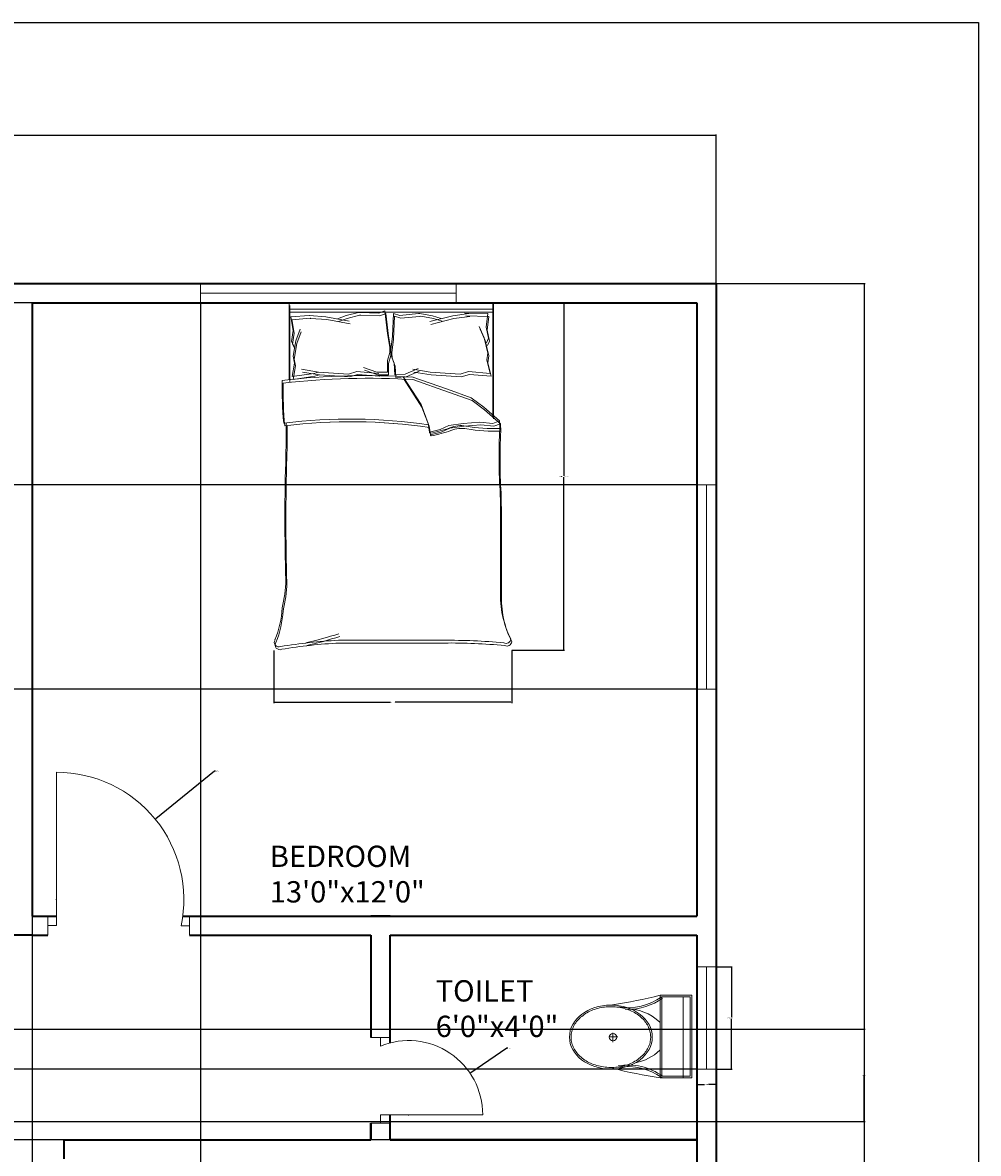
# Model space of a CAD drawing. Units: inches. Extents: x 1861 to 2564, y 1482 to 2317.
# Tile 11 of 11: x 2339 to 2564, y 2051 to 2317. Entities that reach past the tile are written whole.
import ezdxf

# ---------------------------------------------------------------- set-up
doc = ezdxf.new("R2010")
doc.units = ezdxf.units.IN
for name, color, linetype, lineweight in [('A-ANNO-DIMS', 2, 'Continuous', 18), ('A-ANNO-TTLB', 7, 'Continuous', 25), ('A-AREA-IDEN', 7, 'Continuous', 18), ('A-DOOR', 3, 'Continuous', 18), ('A-FLOR-FIXT', 8, 'Continuous', 18), ('A-FURN', 8, 'Continuous', 13), ('A-GLAZ', 4, 'Continuous', 18), ('A-WALL', 7, 'Continuous', 35)]:
    doc.layers.add(name, color=color, linetype=linetype, lineweight=lineweight)
doc.styles.get("Standard").update_dxf_attribs({"font": 'arial.ttf'})
doc.dimstyles.get("Standard").update_dxf_attribs({"dimtxt": 0.18, "dimasz": 0.18, "dimexe": 0.18, "dimexo": 0.0625, "dimgap": 0.09, "dimtad": 0, "dimtih": 1, "dimtoh": 1, "dimdec": 4, "dimzin": 0, "dimdsep": 46, "dimtxsty": 'Standard', "dimcen": 0.09, "dimadec": 0, "dimazin": 0, "dimtfac": 1, "dimtdec": 4, "dimtofl": 0, "dimtmove": 0, "dimatfit": 3, "dimfxl": 1, "dimtolj": 1, "dimtzin": 0, "dimarcsym": 0})

# ---------------------------------------------------------------- blocks, each defined once
blk = doc.blocks.new('A$C31115884')
for p, q in [((257.5, 466.4), (257.5, 523.2)), ((283.1, 497.7), (223.4, 497.7)), ((0, 200), (0, 0)), ((520, 200), (0, 200)), ((10, 190), (10, 10)), ((510, 190), (10, 190)), ((510, 10), (510, 190)), ((520, 0), (520, 200)), ((510, 54.5), (0, 54.5)), ((10, 10), (510, 10)), ((0, 0), (520, 0))]:
    blk.add_line(p, q)
blk.add_circle((255.6, 496.4), 23.6)
for centre, radius, start, end in [((2777.7, -204.6), 2807, 165.4549, 171.71327), ((3237, 905), 2807, 188.28673, 194.5451), ((-294.5, 403.3), 364.7, 324.20913, 9.34987), ((-294.5, 403.3), 374.7, 324.20913, 9.34987), ((805.8, 403.3), 364.7, 170.65013, 215.79087), ((139.5, 406.2), 293.5, 315.84364, 2.65635), ((805.8, 403.3), 374.7, 179.20365, 215.79087), ((383.6, 406.2), 293.5, 190.27735, 224.15636)]:
    blk.add_arc(centre, radius, start, end)
blk.add_ellipse((256.2, 509.9), major_axis=(0, -260.7), ratio=0.772727)
blk.add_open_spline([(256.2, 259.2), (263.1, 259.2), (270, 259.7), (287.8, 262.3), (298.7, 265.1), (319.9, 273.1), (330.2, 278.4), (350.1, 291.1), (359.7, 298.7), (377.7, 315.9), (386.2, 325.5), (401.7, 346.6), (408.8, 358.1), (421.3, 382.5), (426.8, 395.5), (435.9, 422.4), (439.5, 436.4), (444.8, 465.1), (446.5, 479.7), (447.9, 509.2), (447.6, 524), (445, 553.3), (442.7, 567.8), (436.3, 596), (432.1, 609.7), (421.9, 636), (416, 648.6), (402.5, 672.1), (395, 683), (378.6, 703), (369.8, 712.1), (351.1, 728), (341.3, 734.8), (320.9, 746.2), (310.4, 750.7), (288.9, 757.3), (278, 759.4), (256, 761), (245, 760.6), (223.1, 757.2), (212.3, 754.3), (191.1, 746.1), (180.8, 740.7), (160.9, 727.8), (151.4, 720.1), (133.5, 702.7), (125.1, 693), (109.6, 671.7), (102.6, 660.2), (90.2, 635.7), (84.9, 622.7), (76, 595.6), (72.4, 581.6), (67.2, 552.9), (65.6, 538.2), (64.4, 508.8), (64.8, 494), (67.5, 464.7), (69.9, 450.2), (76.6, 422), (80.8, 408.3), (91.1, 382.2), (97.2, 369.7), (110.8, 346.3), (118.4, 335.4), (134.8, 315.6), (143.7, 306.7), (162.4, 290.9), (172.3, 284.2), (192.8, 273), (203.3, 268.6), (224.8, 262.2), (235.8, 260.2), (249.9, 259.3), (253, 259.2), (256.2, 259.2)], degree=3, knots=[0, 0, 0, 0, 0.110105, 0.110105, 0.285049, 0.285049, 0.459994, 0.459994, 0.634938, 0.634938, 0.809882, 0.809882, 0.984827, 0.984827, 1.159771, 1.159771, 1.334715, 1.334715, 1.50966, 1.50966, 1.684604, 1.684604, 1.859549, 1.859549, 2.034493, 2.034493, 2.209437, 2.209437, 2.384382, 2.384382, 2.559326, 2.559326, 2.73427, 2.73427, 2.909215, 2.909215, 3.084159, 3.084159, 3.259103, 3.259103, 3.434048, 3.434048, 3.608992, 3.608992, 3.783936, 3.783936, 3.958881, 3.958881, 4.133825, 4.133825, 4.30877, 4.30877, 4.483714, 4.483714, 4.658658, 4.658658, 4.833603, 4.833603, 5.008547, 5.008547, 5.183491, 5.183491, 5.358436, 5.358436, 5.53338, 5.53338, 5.708324, 5.708324, 5.883269, 5.883269, 6.058213, 6.058213, 6.233158, 6.233158, 6.283185, 6.283185, 6.283185, 6.283185])
blk = doc.blocks.new('WIN-24IN')
for p, q in [((0, 24), (4.5, 24)), ((4.5, 24), (2.25, 24)), ((2.25, 24), (2.25, 0)), ((2.25, 0), (0, 0)), ((0, 0), (4.5, 0))]:
    blk.add_line(p, q)
blk = doc.blocks.new('WIN-60IN')
for p, q in [((0, 4.5), (0, 0)), ((60, 2.25), (60, 4.5)), ((60, 4.5), (60, 0)), ((0, 0), (0, 2.25)), ((0, 2.25), (60, 2.25))]:
    blk.add_line(p, q)
blk = doc.blocks.new('BED-DOUBLE')
for p, q in [((3.48, 63.34), (3.48, 81.45)), ((3.48, 63.34), (3.48, 81.45)), ((51.27, 81.45), (3.48, 81.45)), ((3.48, 79.91), (51.27, 79.91)), ((3.48, 79.91), (51.27, 79.91)), ((3.7, 62.7), (3.7, 80.81)), ((3.7, 62.7), (3.7, 80.81)), ((51.27, 81.45), (51.27, 54.84)), ((51.27, 81.45), (51.27, 54.84)), ((51.27, 81.45), (51.49, 81.45)), ((51.49, 81.45), (51.49, 80.81)), ((51.49, 80.81), (51.49, 54.2)), ((51.49, 80.81), (51.49, 54.2)), ((3.7, 79.27), (51.49, 79.27)), ((3.7, 79.27), (51.49, 79.27)), ((3.9, 78.11), (8.18, 78.44)), ((3.9, 78.11), (8.18, 78.44)), ((3.9, 78.13), (4.47, 74.95)), ((3.9, 78.13), (4.47, 74.95)), ((4.12, 77.49), (4.7, 74.31)), ((4.12, 77.49), (4.7, 74.31)), ((4.13, 77.47), (8.41, 77.8)), ((4.13, 77.47), (8.41, 77.8)), ((8.18, 78.44), (8.29, 78.42)), ((8.18, 78.44), (8.29, 78.42)), ((8.29, 78.42), (12.11, 78.13)), ((8.29, 78.42), (12.11, 78.13)), ((8.41, 77.8), (8.51, 77.78)), ((8.41, 77.8), (8.51, 77.78)), ((8.51, 77.78), (12.34, 77.49)), ((8.51, 77.78), (12.34, 77.49)), ((12.11, 78.13), (17.6, 77.12)), ((12.11, 78.13), (17.6, 77.12)), ((12.34, 77.49), (17.83, 76.48)), ((12.34, 77.49), (17.83, 76.48)), ((14.86, 77.7), (16.88, 78.42)), ((14.86, 77.7), (16.88, 78.42)), ((15.08, 77.06), (17.11, 77.78)), ((15.08, 77.06), (17.11, 77.78)), ((16.88, 78.42), (19.77, 79.14)), ((16.88, 78.42), (19.77, 79.14)), ((17.11, 77.78), (20, 78.5)), ((17.11, 77.78), (20, 78.5)), ((19.77, 79.14), (20.09, 79.14)), ((19.77, 79.14), (20.09, 79.14)), ((20, 78.5), (20.32, 78.5)), ((20, 78.5), (20.32, 78.5)), ((20.09, 79.14), (24.54, 79)), ((20.09, 79.14), (24.54, 79)), ((20.32, 78.5), (24.77, 78.36)), ((20.32, 78.5), (24.77, 78.36)), ((24.54, 79), (25.98, 79.58)), ((24.54, 79), (25.98, 79.58)), ((24.77, 78.36), (26.21, 78.94)), ((24.77, 78.36), (26.21, 78.94)), ((25.98, 79.58), (26.56, 74.23)), ((25.98, 79.58), (26.56, 74.23)), ((26.21, 78.94), (26.79, 73.59)), ((26.21, 78.94), (26.79, 73.59)), ((27.98, 78.95), (27.73, 73.58)), ((27.98, 78.95), (27.73, 73.58)), ((28.21, 78.31), (27.96, 72.94)), ((28.21, 78.31), (27.96, 72.94)), ((29.46, 78.47), (27.98, 78.95)), ((29.46, 78.47), (27.98, 78.95)), ((29.69, 77.83), (28.21, 78.31)), ((29.68, 77.83), (28.21, 78.31)), ((33.88, 78.89), (29.46, 78.47)), ((33.88, 78.89), (29.46, 78.47)), ((34.11, 78.25), (29.68, 77.83)), ((34.11, 78.25), (29.69, 77.83)), ((34.21, 78.91), (33.88, 78.89)), ((34.21, 78.91), (33.88, 78.89)), ((34.43, 78.27), (34.11, 78.25)), ((34.43, 78.27), (34.11, 78.25)), ((37.14, 78.37), (34.21, 78.91)), ((37.14, 78.37), (34.21, 78.91)), ((37.36, 77.73), (34.43, 78.27)), ((37.36, 77.73), (34.43, 78.27)), ((41.92, 78.38), (36.5, 77.02)), ((41.92, 78.38), (36.5, 77.02)), ((42.14, 77.74), (36.72, 76.38)), ((42.14, 77.74), (36.72, 76.38)), ((39.2, 77.77), (37.14, 78.37)), ((39.2, 77.77), (37.14, 78.37)), ((39.43, 77.13), (37.36, 77.73)), ((39.43, 77.13), (37.36, 77.73)), ((45.71, 78.9), (41.92, 78.38)), ((45.71, 78.9), (41.92, 78.38)), ((45.94, 78.26), (42.14, 77.74)), ((45.94, 78.26), (42.14, 77.74)), ((50.11, 78.89), (44.71, 78.99)), ((44.71, 78.99), (45.71, 78.9)), ((50.11, 78.89), (44.71, 78.99)), ((44.71, 78.99), (45.71, 78.9)), ((50.34, 78.25), (44.94, 78.35)), ((44.94, 78.35), (45.94, 78.26)), ((50.34, 78.25), (44.94, 78.35)), ((44.94, 78.35), (45.94, 78.26)), ((50.11, 78.89), (49.73, 75.68)), ((50.11, 78.89), (49.73, 75.68)), ((50.34, 78.25), (49.96, 75.04)), ((50.34, 78.25), (49.96, 75.04)), ((4.47, 74.95), (4.04, 72.35)), ((4.47, 74.95), (4.04, 72.35)), ((5.05, 72.49), (6.06, 75.24)), ((5.05, 72.49), (6.06, 75.24)), ((5.28, 71.85), (6.29, 74.6)), ((5.28, 71.85), (6.29, 74.6)), ((49.31, 73.19), (48.13, 75.87)), ((49.31, 73.19), (48.13, 75.87)), ((49.54, 72.55), (48.36, 75.23)), ((49.54, 72.55), (48.36, 75.23)), ((49.73, 75.68), (50.33, 73.11)), ((49.73, 75.68), (50.33, 73.11)), ((49.96, 75.04), (50.56, 72.47)), ((49.96, 75.04), (50.56, 72.47)), ((4.04, 72.35), (4.62, 71.33)), ((4.04, 72.35), (4.62, 71.33)), ((4.7, 74.31), (4.27, 71.71)), ((4.7, 74.31), (4.27, 71.71)), ((4.27, 71.71), (4.85, 70.69)), ((4.27, 71.71), (4.85, 70.69)), ((4.47, 68.88), (5.05, 72.49)), ((4.47, 68.88), (5.05, 72.49)), ((4.7, 68.24), (5.28, 71.85)), ((4.7, 68.24), (5.28, 71.85)), ((26.56, 74.23), (27.14, 71.04)), ((26.56, 74.23), (27.14, 71.04)), ((26.79, 73.59), (27.37, 70.41)), ((26.79, 73.59), (27.37, 70.41)), ((27.73, 73.58), (27.36, 70.37)), ((27.73, 73.58), (27.36, 70.37)), ((27.96, 72.94), (27.58, 69.73)), ((27.96, 72.94), (27.58, 69.73)), ((50.11, 69.62), (49.31, 73.19)), ((50.11, 69.62), (49.31, 73.19)), ((50.34, 68.98), (49.54, 72.55)), ((50.34, 68.98), (49.54, 72.55)), ((50.33, 73.11), (49.82, 72.06)), ((50.33, 73.11), (49.82, 72.06)), ((50.56, 72.47), (50.04, 71.42)), ((50.56, 72.47), (50.04, 71.42)), ((27.14, 69.74), (26.56, 67.86)), ((27.14, 69.74), (26.56, 67.86)), ((27.37, 69.1), (26.79, 67.22)), ((27.37, 69.1), (26.79, 67.22)), ((27.14, 71.04), (27.14, 69.74)), ((27.14, 71.04), (27.14, 69.74)), ((27.36, 70.37), (27.44, 69.07)), ((27.36, 70.37), (27.44, 69.07)), ((27.37, 70.41), (27.37, 69.1)), ((27.37, 70.41), (27.37, 69.1)), ((27.44, 69.07), (28.13, 67.23)), ((27.44, 69.07), (28.13, 67.23)), ((27.58, 69.73), (27.67, 68.43)), ((27.58, 69.73), (27.67, 68.43)), ((49.92, 68.01), (50.11, 69.62)), ((49.92, 68.01), (50.11, 69.62)), ((4.18, 64.1), (4.76, 67.29)), ((4.18, 64.1), (4.76, 67.29)), ((4.41, 63.46), (4.99, 66.65)), ((4.41, 63.46), (4.99, 66.65)), ((4.76, 67.29), (4.47, 68.88)), ((4.76, 67.29), (4.47, 68.88)), ((4.99, 66.65), (4.7, 68.24)), ((4.99, 66.65), (4.7, 68.24)), ((26.56, 67.86), (26.56, 65.18)), ((26.56, 67.86), (26.56, 65.18)), ((26.79, 67.22), (26.79, 64.54)), ((26.79, 67.22), (26.79, 64.54)), ((27.67, 68.43), (28.36, 66.59)), ((27.67, 68.43), (28.36, 66.59)), ((28.13, 67.23), (28.3, 64.55)), ((28.13, 67.23), (28.3, 64.55)), ((28.36, 66.59), (28.53, 63.91)), ((28.36, 66.59), (28.53, 63.91)), ((50.7, 64.87), (49.92, 68.01)), ((50.7, 64.87), (49.92, 68.01)), ((50.15, 67.37), (50.34, 68.98)), ((50.15, 67.37), (50.34, 68.98)), ((50.93, 64.23), (50.15, 67.37)), ((50.93, 64.23), (50.15, 67.37)), ((9.28, 64.83), (4.18, 64.1)), ((9.28, 64.83), (4.18, 64.1)), ((9.51, 64.19), (4.41, 63.46)), ((9.51, 64.19), (4.41, 63.46)), ((6.38, 65.82), (10.41, 65.15)), ((6.38, 65.82), (10.41, 65.15)), ((6.61, 65.18), (10.64, 64.51)), ((6.61, 65.18), (10.64, 64.51)), ((10.41, 65.15), (9.28, 64.83)), ((10.41, 65.15), (9.28, 64.83)), ((10.64, 64.51), (9.51, 64.19)), ((10.64, 64.51), (9.51, 64.19)), ((10.41, 65.15), (17.42, 64.72)), ((10.41, 65.15), (17.42, 64.72)), ((10.64, 64.51), (17.65, 64.08)), ((10.64, 64.51), (17.65, 64.08)), ((17.42, 64.72), (19.38, 65.28)), ((17.42, 64.72), (19.38, 65.28)), ((17.65, 64.08), (19.61, 64.64)), ((17.65, 64.08), (19.61, 64.64)), ((19.38, 65.28), (24.52, 64.87)), ((19.38, 65.28), (24.52, 64.87)), ((19.61, 64.64), (24.75, 64.23)), ((19.61, 64.64), (24.74, 64.23)), ((24.1, 65.18), (20.96, 66.27)), ((24.1, 65.18), (20.96, 66.27)), ((24.33, 64.54), (21.19, 65.63)), ((24.33, 64.54), (21.19, 65.63)), ((26.56, 65.18), (24.1, 65.18)), ((26.56, 65.18), (24.1, 65.18)), ((26.79, 64.54), (24.33, 64.54)), ((26.79, 64.54), (24.33, 64.54)), ((28.3, 64.55), (30.75, 64.71)), ((28.3, 64.55), (30.75, 64.71)), ((28.53, 63.91), (30.98, 64.07)), ((28.53, 63.91), (30.98, 64.07)), ((30.26, 64.06), (34.45, 57.57)), ((30.26, 64.06), (34.45, 57.57)), ((30.75, 64.71), (33.82, 65.99)), ((30.75, 64.71), (33.82, 65.99)), ((30.98, 64.07), (34.05, 65.35)), ((30.98, 64.07), (34.05, 65.35)), ((40.65, 61.13), (32.31, 64.06)), ((40.64, 61.13), (32.31, 64.06)), ((32.56, 65.82), (36.6, 65.15)), ((32.57, 65.82), (36.6, 65.15)), ((32.79, 65.18), (36.83, 64.51)), ((32.79, 65.18), (36.83, 64.51)), ((36.6, 65.15), (43.61, 64.72)), ((36.6, 65.15), (43.61, 64.72)), ((36.83, 64.51), (43.84, 64.08)), ((36.83, 64.51), (43.84, 64.08)), ((43.61, 64.72), (45.57, 65.28)), ((43.61, 64.72), (45.57, 65.28)), ((43.84, 64.08), (45.8, 64.64)), ((43.84, 64.08), (45.8, 64.64)), ((45.57, 65.28), (50.7, 64.87)), ((45.57, 65.28), (50.7, 64.87)), ((45.8, 64.64), (50.93, 64.23)), ((45.8, 64.64), (50.93, 64.23)), ((30.49, 63.42), (34.68, 56.93)), ((30.49, 63.42), (34.68, 56.93)), ((40.87, 60.49), (32.54, 63.42)), ((40.87, 60.49), (32.54, 63.42)), ((46.22, 59.12), (40.64, 61.13)), ((46.22, 59.12), (40.65, 61.13)), ((46.45, 58.48), (40.87, 60.49)), ((46.45, 58.48), (40.87, 60.49)), ((49.16, 56.95), (46.22, 59.12)), ((49.16, 56.95), (46.22, 59.12)), ((49.39, 56.31), (46.45, 58.48)), ((49.39, 56.31), (46.45, 58.48)), ((34.45, 57.57), (36.15, 53.08)), ((34.45, 57.57), (36.15, 53.08)), ((34.68, 56.93), (36.38, 52.44)), ((34.68, 56.93), (36.38, 52.44)), ((52.87, 53.7), (49.16, 56.95)), ((52.87, 53.7), (49.16, 56.95)), ((53.1, 53.06), (49.39, 56.31)), ((53.1, 53.06), (49.39, 56.31)), ((44.36, 53.08), (48.23, 53.39)), ((44.36, 53.08), (48.23, 53.39)), ((48.23, 53.39), (51.33, 53.08)), ((48.23, 53.39), (51.33, 53.08)), ((51.33, 53.08), (52.87, 53.7)), ((51.33, 53.08), (52.87, 53.7)), ((52.95, 51.95), (52.87, 53.7, 3.87)), ((52.95, 51.95), (52.87, 53.7, 3.87)), ((36.15, 53.08), (36.46, 51.07)), ((36.15, 53.08), (36.46, 51.07)), ((36.38, 52.44), (36.69, 50.43)), ((36.38, 52.44), (36.69, 50.43)), ((36.46, 51.07), (38.94, 51.69)), ((36.46, 51.07), (38.94, 51.69)), ((36.69, 50.43), (39.17, 51.05)), ((36.69, 50.43), (39.17, 51.05)), ((38.94, 51.69), (40.95, 52.62)), ((38.94, 51.69), (40.95, 52.62)), ((39.17, 51.05), (41.18, 51.98)), ((39.17, 51.05), (41.18, 51.98)), ((40.95, 52.62), (44.36, 53.08)), ((40.95, 52.62), (44.36, 53.08)), ((41.18, 51.98), (44.59, 52.44)), ((41.18, 51.98), (44.59, 52.44)), ((44.59, 52.44), (48.46, 52.75)), ((44.59, 52.44), (48.46, 52.75)), ((48.46, 52.75), (51.56, 52.44)), ((48.46, 52.75), (51.56, 52.44)), ((51.56, 52.44), (53.1, 53.06)), ((51.56, 52.44), (53.1, 53.06)), ((53.18, 51.32), (53.1, 53.06, 3.87)), ((53.18, 51.32), (53.1, 53.06, 3.87)), ((15.06, 2.2), (39.68, 2.2)), ((15.06, 2.2), (39.68, 2.2)), ((15.29, 1.56), (39.91, 1.56)), ((15.29, 1.56), (39.91, 1.56))]:
    blk.add_line(p, q)
for centre, radius, start, end in [((21.36, -100.61), 164.97, 86.0865, 96.7821), ((21.36, -100.61), 164.97, 86.0865, 96.7821), ((21.59, -101.25), 164.97, 86.0865, 96.7821), ((21.59, -101.25), 164.97, 86.0865, 96.7821), ((85.16, 61.35), 83.31, 178.7218, 185.604), ((85.16, 61.35), 83.31, 178.7218, 185.604), ((85.39, 60.71), 83.31, 178.7218, 185.604), ((85.39, 60.71), 83.31, 178.7218, 185.604), ((17.76, -74.87), 129.02, 81.7845, 96.9006), ((17.76, -74.87), 129.02, 81.7845, 96.9006), ((17.99, -75.51), 129.02, 81.7845, 96.9006), ((17.98, -75.51), 129.02, 81.7845, 96.9006), ((-167.31, 50.27), 170.11, 358.4762, 1.0082), ((-167.31, 50.27), 170.11, 358.4762, 1.0082), ((-167.08, 49.63), 170.11, 358.4762, 1.0082), ((-167.08, 49.63), 170.11, 358.4762, 1.0082), ((36.64, 51.01), 0.185, 160.2464, 271.1377), ((36.64, 51.01), 0.185, 160.2464, 271.1377), ((31.15, 79.96), 29.65, 280.6617, 289.8806), ((31.15, 79.96), 29.65, 280.6617, 289.8806), ((31.38, 79.32), 29.65, 280.6617, 289.8806), ((31.38, 79.32), 29.65, 280.6617, 289.8806), ((43.74, 46.38), 6.22, 78.6608, 113.7384), ((43.74, 46.38), 6.22, 78.6608, 113.7384), ((43.97, 45.74), 6.22, 78.6608, 113.7384), ((43.97, 45.74), 6.22, 78.6608, 113.7384), ((51.33, 88.1), 36.18, 259.8763, 272.5657), ((51.33, 88.1), 36.18, 259.8763, 272.5657), ((51.56, 87.46), 36.18, 259.8763, 272.5657), ((51.56, 87.46), 36.18, 259.8763, 272.5657), ((182.27, 45.13), 129.5, 176.9791, 183.8365), ((182.27, 45.13), 129.5, 176.9791, 183.8365), ((182.5, 44.49), 129.5, 176.9791, 183.8365), ((182.49, 44.49), 129.5, 176.9791, 183.8365), ((36.87, 50.37), 0.185, 160.2464, 271.1377), ((36.87, 50.37), 0.185, 160.2464, 271.1377), ((484.82, 30.83), 482.31, 178.2277, 181.7185), ((484.82, 30.83), 482.31, 178.2277, 181.7185), ((485.05, 30.19), 482.31, 178.2277, 181.7185), ((485.05, 30.19), 482.31, 178.2277, 181.7185), ((-4508.74, 13.62), 4561.86, 0.00217, 0.28689), ((-4508.74, 13.62), 4561.86, 0.00217, 0.28689), ((-4508.51, 12.98), 4561.86, 0.00217, 0.28689), ((-4508.51, 12.98), 4561.86, 0.00217, 0.28689), ((-26.9, 16.93), 29.63, 346.0648, 358.9113), ((-26.9, 16.93), 29.63, 346.0648, 358.9113), ((-26.67, 16.29), 29.63, 346.0648, 358.9113), ((-26.67, 16.29), 29.63, 346.0648, 358.9113), ((76.16, 12.78), 23.07, 177.4714, 206.4681), ((76.16, 12.78), 23.07, 177.4714, 206.4681), ((76.39, 12.14), 23.07, 177.4714, 206.4681), ((76.39, 12.14), 23.07, 177.4714, 206.4681), ((-21.66, 11.17), 23.56, 337.9751, 356.652), ((-21.66, 11.17), 23.56, 337.9751, 356.652), ((-21.43, 10.53), 23.56, 337.9751, 356.652), ((-21.43, 10.53), 23.56, 337.9751, 356.652), ((-17.22, 105.16), 106.46, 283.3832, 287.7053), ((-17.22, 105.16), 106.46, 283.3832, 287.7053), ((-16.99, 104.52), 106.46, 283.3832, 287.7053), ((-16.99, 104.52), 106.46, 283.3832, 287.7053), ((1.09, 1.73), 1.09, 146.1736, 293.4781), ((1.09, 1.73), 1.09, 146.1736, 293.4781), ((1.32, 1.09), 1.09, 146.1736, 293.4781), ((1.32, 1.09), 1.09, 146.1736, 293.4781), ((21.43, -119.39), 121.76, 92.9958, 99.4091), ((21.43, -119.39), 121.76, 92.9958, 99.4091), ((21.66, -120.03), 121.76, 92.9958, 99.4091), ((21.66, -120.03), 121.76, 92.9958, 99.4091), ((41.15, -130.83), 133.04, 84.4998, 90.6351), ((41.15, -130.83), 133.04, 84.4998, 90.6351), ((41.38, -131.47), 133.04, 84.4998, 90.6351), ((41.38, -131.47), 133.04, 84.4998, 90.6351), ((54.41, 2.58), 1.1, 242.6588, 356.02), ((54.41, 2.58), 1.1, 242.6588, 356.02), ((54.64, 1.94), 1.1, 242.6588, 356.02), ((54.64, 1.94), 1.1, 242.6588, 356.02)]:
    blk.add_arc(centre, radius, start, end)
blk = doc.blocks.new('*D12')
at = {"layer": 'A-ANNO-DIMS', "color": 0, "lineweight": -2, "transparency": 16777216}
for p, q in [((2454.34, 2250.89), (2466.69, 2250.89)), ((2466.51, 2250.71), (2466.51, 2210.29)), ((2466.51, 2169.52), (2466.51, 2209.93)), ((2454.34, 2169.34), (2466.69, 2169.34))]:
    blk.add_line(p, q, dxfattribs=at)
at = {"layer": 'A-ANNO-DIMS', "color": 0, "transparency": 16777216}
for points in [[(2466.48, 2250.71), (2466.54, 2250.71), (2466.51, 2250.89)], [(2466.48, 2169.52), (2466.54, 2169.52), (2466.51, 2169.34)]]:
    blk.add_solid(points, dxfattribs=at)
at = {"layer": 'Defpoints', "color": 0, "transparency": 16777216}
for p in [(2454.28, 2250.89), (2466.51, 2250.89), (2454.28, 2169.34)]:
    blk.add_point(p, dxfattribs=at)
at = {"layer": 'A-ANNO-DIMS', "color": 0, "transparency": 16777216, "insert": (2466.51, 2210.11), "char_height": 0.18, "attachment_point": 5}
blk.add_mtext('\\A1;DOUBLE BED 82 TYP.', dxfattribs=at)
blk = doc.blocks.new('*D13')
at = {"layer": 'A-ANNO-DIMS', "color": 0, "lineweight": -2, "transparency": 16777216}
for p, q in [((2398.45, 2169.27), (2398.45, 2156.92)), ((2454.28, 2169.27), (2454.28, 2156.92)), ((2398.63, 2157.1), (2425.84, 2157.1)), ((2454.1, 2157.1), (2426.89, 2157.1))]:
    blk.add_line(p, q, dxfattribs=at)
at = {"layer": 'A-ANNO-DIMS', "color": 0, "transparency": 16777216}
for points in [[(2398.63, 2157.13), (2398.63, 2157.07), (2398.45, 2157.1)], [(2454.1, 2157.13), (2454.1, 2157.07), (2454.28, 2157.1)]]:
    blk.add_solid(points, dxfattribs=at)
at = {"layer": 'Defpoints', "color": 0, "transparency": 16777216}
for p in [(2398.45, 2169.34), (2454.28, 2169.34), (2454.28, 2157.1)]:
    blk.add_point(p, dxfattribs=at)
at = {"layer": 'A-ANNO-DIMS', "color": 0, "transparency": 16777216, "insert": (2426.37, 2157.1), "char_height": 0.18, "attachment_point": 5}
blk.add_mtext('\\A1;56 TYP.', dxfattribs=at)
blk = doc.blocks.new('*D16')
at = {"layer": 'A-ANNO-DIMS', "color": 0, "lineweight": -2, "transparency": 16777216}
for p, q in [((2502.3, 2094.96), (2506.02, 2094.96)), ((2505.84, 2094.78), (2505.84, 2083.14)), ((2505.84, 2071.14), (2505.84, 2082.77)), ((2502.3, 2070.96), (2506.02, 2070.96))]:
    blk.add_line(p, q, dxfattribs=at)
at = {"layer": 'A-ANNO-DIMS', "color": 0, "transparency": 16777216}
for points in [[(2505.81, 2094.78), (2505.87, 2094.78), (2505.84, 2094.96)], [(2505.81, 2071.14), (2505.87, 2071.14), (2505.84, 2070.96)]]:
    blk.add_solid(points, dxfattribs=at)
at = {"layer": 'Defpoints', "color": 0, "transparency": 16777216}
for p in [(2502.24, 2094.96), (2505.84, 2094.96), (2502.24, 2070.96)]:
    blk.add_point(p, dxfattribs=at)
at = {"layer": 'A-ANNO-DIMS', "color": 0, "transparency": 16777216, "insert": (2505.84, 2082.96), "char_height": 0.18, "attachment_point": 5}
blk.add_mtext('\\A1;WINDOW 24 TYP.', dxfattribs=at)
blk = doc.blocks.new('*D17')
at = {"layer": 'A-ANNO-DIMS', "color": 0, "lineweight": -2, "transparency": 16777216}
for p, q in [((2497.74, 2070.89), (2497.74, 2067.18)), ((2502.24, 2070.89), (2502.24, 2067.18)), ((2497.92, 2067.36), (2499.53, 2067.36)), ((2502.06, 2067.36), (2500.45, 2067.36))]:
    blk.add_line(p, q, dxfattribs=at)
at = {"layer": 'A-ANNO-DIMS', "color": 0, "transparency": 16777216}
for points in [[(2497.92, 2067.39), (2497.92, 2067.33), (2497.74, 2067.36)], [(2502.06, 2067.39), (2502.06, 2067.33), (2502.24, 2067.36)]]:
    blk.add_solid(points, dxfattribs=at)
at = {"layer": 'Defpoints', "color": 0, "transparency": 16777216}
for p in [(2497.74, 2070.96), (2502.24, 2070.96), (2502.24, 2067.36)]:
    blk.add_point(p, dxfattribs=at)
at = {"layer": 'A-ANNO-DIMS', "color": 0, "transparency": 16777216, "insert": (2499.99, 2067.36), "char_height": 0.18, "attachment_point": 5}
blk.add_mtext('\\A1;5 TYP.', dxfattribs=at)
blk = doc.blocks.new('*D34')
at = {"layer": 'A-ANNO-DIMS', "color": 0, "lineweight": -2, "transparency": 16777216}
for p, q in [((1927.74, 2255.45), (1927.74, 2290.37)), ((1927.92, 2290.19), (2214.59, 2290.19)), ((2502.06, 2290.19), (2215.38, 2290.19)), ((2502.24, 2255.45), (2502.24, 2290.37))]:
    blk.add_line(p, q, dxfattribs=at)
at = {"layer": 'A-ANNO-DIMS', "color": 0, "transparency": 16777216}
for points in [[(1927.92, 2290.22), (1927.92, 2290.16), (1927.74, 2290.19)], [(2502.06, 2290.22), (2502.06, 2290.16), (2502.24, 2290.19)]]:
    blk.add_solid(points, dxfattribs=at)
at = {"layer": 'Defpoints', "color": 0, "transparency": 16777216}
for p in [(2502.24, 2290.19), (1927.74, 2255.39), (2502.24, 2255.39)]:
    blk.add_point(p, dxfattribs=at)
at = {"layer": 'A-ANNO-DIMS', "color": 0, "transparency": 16777216, "insert": (2214.99, 2290.19), "char_height": 0.18, "attachment_point": 5}
blk.add_mtext('\\A1;574.5', dxfattribs=at)
blk = doc.blocks.new('*D38')
at = {"layer": 'A-ANNO-DIMS', "color": 0, "lineweight": -2, "transparency": 16777216}
for p, q in [((2341.74, 2250.82), (2341.74, 1545.6)), ((2381.24, 2250.82), (2381.24, 1545.6)), ((2341.92, 1545.78), (2361.16, 1545.78)), ((2381.06, 1545.78), (2361.81, 1545.78))]:
    blk.add_line(p, q, dxfattribs=at)
at = {"layer": 'A-ANNO-DIMS', "color": 0, "transparency": 16777216}
for points in [[(2341.92, 1545.81), (2341.92, 1545.75), (2341.74, 1545.78)], [(2381.06, 1545.81), (2381.06, 1545.75), (2381.24, 1545.78)]]:
    blk.add_solid(points, dxfattribs=at)
at = {"layer": 'Defpoints', "color": 0, "transparency": 16777216}
for p in [(2341.74, 2250.89), (2381.24, 2250.89), (2381.24, 1545.78)]:
    blk.add_point(p, dxfattribs=at)
at = {"layer": 'A-ANNO-DIMS', "color": 0, "transparency": 16777216, "insert": (2361.49, 1545.78), "char_height": 0.18, "attachment_point": 5}
blk.add_mtext('\\A1;39.5', dxfattribs=at)
blk = doc.blocks.new('*D45')
at = {"layer": 'A-ANNO-DIMS', "color": 0, "lineweight": -2, "transparency": 16777216}
for p, q in [((2502.3, 2255.39), (2537.22, 2255.39)), ((2537.04, 2255.21), (2537.04, 1951.82)), ((2537.04, 1648.07), (2537.04, 1951.45)), ((2473.32, 1647.89), (2537.22, 1647.89))]:
    blk.add_line(p, q, dxfattribs=at)
at = {"layer": 'A-ANNO-DIMS', "color": 0, "transparency": 16777216}
for points in [[(2537.01, 2255.21), (2537.07, 2255.21), (2537.04, 2255.39)], [(2537.01, 1648.07), (2537.07, 1648.07), (2537.04, 1647.89)]]:
    blk.add_solid(points, dxfattribs=at)
at = {"layer": 'Defpoints', "color": 0, "transparency": 16777216}
for p in [(2502.24, 2255.39), (2537.04, 2255.39), (2473.26, 1647.89)]:
    blk.add_point(p, dxfattribs=at)
at = {"layer": 'A-ANNO-DIMS', "color": 0, "transparency": 16777216, "insert": (2537.04, 1951.64), "char_height": 0.18, "attachment_point": 5}
blk.add_mtext('\\A1;607.5', dxfattribs=at)
blk = doc.blocks.new('*D60')
at = {"layer": 'A-ANNO-DIMS', "color": 0, "lineweight": -2, "transparency": 16777216}
for p, q in [((2497.68, 2208.17), (1892.76, 2208.17)), ((1892.94, 2207.99), (1892.94, 2184.35)), ((1892.94, 2160.35), (1892.94, 2183.99)), ((2497.68, 2160.17), (1892.76, 2160.17))]:
    blk.add_line(p, q, dxfattribs=at)
at = {"layer": 'A-ANNO-DIMS', "color": 0, "transparency": 16777216}
for points in [[(1892.91, 2207.99), (1892.97, 2207.99), (1892.94, 2208.17)], [(1892.91, 2160.35), (1892.97, 2160.35), (1892.94, 2160.17)]]:
    blk.add_solid(points, dxfattribs=at)
at = {"layer": 'Defpoints', "color": 0, "transparency": 16777216}
for p in [(1892.94, 2208.17), (2497.74, 2208.17), (2497.74, 2160.17)]:
    blk.add_point(p, dxfattribs=at)
at = {"layer": 'A-ANNO-DIMS', "color": 0, "transparency": 16777216, "insert": (1892.94, 2184.17), "char_height": 0.18, "attachment_point": 5}
blk.add_mtext('\\A1;48', dxfattribs=at)
blk = doc.blocks.new('*D61')
at = {"layer": 'A-ANNO-DIMS', "color": 0, "lineweight": -2, "transparency": 16777216}
for p, q in [((2008.8, 2080.33), (2537.22, 2080.33)), ((2537.04, 2080.15), (2537.04, 2069.66)), ((2537.04, 2058.82), (2537.04, 2069.3)), ((2008.8, 2058.64), (2537.22, 2058.64))]:
    blk.add_line(p, q, dxfattribs=at)
at = {"layer": 'A-ANNO-DIMS', "color": 0, "transparency": 16777216}
for points in [[(2537.01, 2080.15), (2537.07, 2080.15), (2537.04, 2080.33)], [(2537.01, 2058.82), (2537.07, 2058.82), (2537.04, 2058.64)]]:
    blk.add_solid(points, dxfattribs=at)
at = {"layer": 'Defpoints', "color": 0, "transparency": 16777216}
for p in [(2008.74, 2080.33), (2537.04, 2080.33), (2008.74, 2058.64)]:
    blk.add_point(p, dxfattribs=at)
at = {"layer": 'A-ANNO-DIMS', "color": 0, "transparency": 16777216, "insert": (2537.04, 2069.48), "char_height": 0.18, "attachment_point": 5}
blk.add_mtext('\\A1;21.693', dxfattribs=at)
blk = doc.blocks.new('*D63')
at = {"layer": 'A-ANNO-DIMS', "color": 0, "lineweight": -2, "transparency": 16777216}
for p, q in [((2497.68, 2250.89), (1892.76, 2250.89)), ((1892.94, 2250.71), (1892.94, 2229.71)), ((1892.94, 2208.35), (1892.94, 2229.35)), ((2497.68, 2208.17), (1892.76, 2208.17))]:
    blk.add_line(p, q, dxfattribs=at)
at = {"layer": 'A-ANNO-DIMS', "color": 0, "transparency": 16777216}
for points in [[(1892.91, 2250.71), (1892.97, 2250.71), (1892.94, 2250.89)], [(1892.91, 2208.35), (1892.97, 2208.35), (1892.94, 2208.17)]]:
    blk.add_solid(points, dxfattribs=at)
at = {"layer": 'Defpoints', "color": 0, "transparency": 16777216}
for p in [(2497.74, 2250.89), (1892.94, 2208.17), (2497.74, 2208.17)]:
    blk.add_point(p, dxfattribs=at)
at = {"layer": 'A-ANNO-DIMS', "color": 0, "transparency": 16777216, "insert": (1892.94, 2229.53), "char_height": 0.18, "attachment_point": 5}
blk.add_mtext('\\A1;42.71', dxfattribs=at)
blk = doc.blocks.new('*D64')
at = {"layer": 'A-ANNO-DIMS', "color": 0, "lineweight": -2, "transparency": 16777216}
for p, q in [((2497.68, 2070.96), (1892.76, 2070.96)), ((1892.94, 2070.78), (1892.94, 2062.85)), ((1892.94, 2054.57), (1892.94, 2062.49)), ((2497.68, 2054.39), (1892.76, 2054.39))]:
    blk.add_line(p, q, dxfattribs=at)
at = {"layer": 'A-ANNO-DIMS', "color": 0, "transparency": 16777216}
for points in [[(1892.91, 2070.78), (1892.97, 2070.78), (1892.94, 2070.96)], [(1892.91, 2054.57), (1892.97, 2054.57), (1892.94, 2054.39)]]:
    blk.add_solid(points, dxfattribs=at)
at = {"layer": 'Defpoints', "color": 0, "transparency": 16777216}
for p in [(2497.74, 2070.96), (1892.94, 2054.39), (2497.74, 2054.39)]:
    blk.add_point(p, dxfattribs=at)
at = {"layer": 'A-ANNO-DIMS', "color": 0, "transparency": 16777216, "insert": (1892.94, 2062.67), "char_height": 0.18, "attachment_point": 5}
blk.add_mtext('\\A1;16.57', dxfattribs=at)
blk = doc.blocks.new('*D78')
at = {"layer": 'A-ANNO-DIMS', "color": 0, "lineweight": -2, "transparency": 16777216}
for p, q in [((2384.56, 2140.93), (2370.77, 2129.73)), ((2384.74, 2140.93), (2384.56, 2140.93)), ((2347.33, 2110.77), (2347.51, 2110.77)), ((2347.42, 2110.68), (2347.42, 2110.86))]:
    blk.add_line(p, q, dxfattribs=at)
at = {"layer": 'A-ANNO-DIMS', "color": 0, "transparency": 16777216}
blk.add_solid([(2370.75, 2129.75), (2370.79, 2129.71), (2370.63, 2129.62)], dxfattribs=at)
at = {"layer": 'Defpoints', "color": 0, "transparency": 16777216}
for p in [(2370.63, 2129.62), (2347.42, 2110.77)]:
    blk.add_point(p, dxfattribs=at)
at = {"layer": 'A-ANNO-DIMS', "color": 0, "transparency": 16777216, "insert": (2385.15, 2140.93), "char_height": 0.18, "attachment_point": 5}
blk.add_mtext('\\A1;R29.9', dxfattribs=at)
blk = doc.blocks.new('*D91')
at = {"layer": 'A-ANNO-DIMS', "color": 0, "lineweight": -2, "transparency": 16777216}
for p, q in [((2453.17, 2075.86), (2444.65, 2070.1)), ((2453.35, 2075.86), (2453.17, 2075.86)), ((2429.97, 2060.24), (2430.15, 2060.24)), ((2430.06, 2060.15), (2430.06, 2060.33))]:
    blk.add_line(p, q, dxfattribs=at)
at = {"layer": 'A-ANNO-DIMS', "color": 0, "transparency": 16777216}
blk.add_solid([(2444.63, 2070.13), (2444.67, 2070.08), (2444.5, 2070)], dxfattribs=at)
at = {"layer": 'Defpoints', "color": 0, "transparency": 16777216}
for p in [(2444.5, 2070), (2430.06, 2060.24)]:
    blk.add_point(p, dxfattribs=at)
at = {"layer": 'A-ANNO-DIMS', "color": 0, "transparency": 16777216, "insert": (2453.83, 2075.86), "char_height": 0.18, "attachment_point": 5}
blk.add_mtext('\\A1;R17.43', dxfattribs=at)

msp = doc.modelspace()

# ---------------------------------------------------------------- linework, layer by layer
at = {"layer": 'A-ANNO-TTLB'}
msp.add_lwpolyline([(1861.1332, 2316.6589), (2563.8077, 2316.6589), (2563.8077, 1482.0728), (1861.1332, 1482.0728)], close=True, dxfattribs=at)
at = {"layer": 'A-DOOR'}
for p, q in [((2347.422, 2104.6664), (2347.422, 2140.6664)), ((2345.422, 2106.8854), (2345.422, 2103.5496)), ((2378.6849, 2106.8854), (2378.6849, 2102.3854)), ((2345.422, 2102.3854), (2345.422, 2104.6664)), ((2345.422, 2104.6664), (2347.422, 2104.6664)), ((2345.422, 2103.5496), (2345.422, 2102.3854)), ((2378.6849, 2104.6354), (2376.6849, 2104.6354)), ((2378.6849, 2102.3854), (2378.6849, 2104.6354)), ((2421.2393, 2078.3854), (2425.7393, 2078.3854)), ((2425.7393, 2078.3854), (2423.4893, 2078.3854)), ((2423.4893, 2078.3854), (2423.4893, 2076.3854)), ((2423.4893, 2058.2408), (2423.4893, 2060.2408)), ((2423.4893, 2060.2408), (2447.4893, 2060.2408)), ((2421.2393, 2058.2408), (2425.7393, 2058.2408)), ((2425.7393, 2058.2408), (2421.2393, 2058.2408)), ((2421.2393, 2058.2408), (2423.4893, 2058.2408))]:
    msp.add_line(p, q, dxfattribs=at)
for centre, radius, start, end in [((2347.422, 2110.7678), 29.8986, 348.164205, 90), ((2430.0591, 2060.2408), 17.4302, 360, 112.143263)]:
    msp.add_arc(centre, radius, start, end, dxfattribs=at)
at = {"layer": 'A-GLAZ'}
for p, q in [((2497.7393, 2208.1728), (2502.2393, 2208.1728)), ((2502.2393, 2208.1728), (2499.9893, 2208.1728)), ((2499.9893, 2208.1728), (2499.9893, 2160.1728)), ((2499.9893, 2160.1728), (2497.7393, 2160.1728)), ((2497.7393, 2160.1728), (2502.2393, 2160.1728))]:
    msp.add_line(p, q, dxfattribs=at)
at = {"layer": 'A-WALL'}
for p, q in [((1927.7393, 2255.3854), (2502.2393, 2255.3854)), ((2502.2393, 2255.3854), (2502.2393, 1700.3854)), ((2341.7393, 2250.8854), (2341.7393, 2106.8854)), ((2341.7393, 2250.8854), (2497.7393, 2250.8854)), ((2497.7393, 2250.8854), (2497.7393, 2106.8854)), ((2341.7393, 2106.8854), (2347.422, 2106.8854)), ((2377.0674, 2106.8854), (2497.7393, 2106.8854)), ((2425.7393, 2106.8854), (2421.2393, 2106.8854)), ((2341.7393, 2102.3854), (2337.2393, 2102.3854)), ((2341.7393, 2102.3854), (2345.422, 2102.3854)), ((2378.6849, 2102.3854), (2421.2393, 2102.3854)), ((2421.2393, 2102.3854), (2421.2393, 2078.3854)), ((2425.7393, 2077.1272), (2425.7393, 2102.3854)), ((2425.7393, 2102.3854), (2497.7393, 2102.3854)), ((2497.7393, 2102.3854), (2497.7393, 1905.8854)), ((2425.7393, 2054.3854), (2425.7393, 2060.2408)), ((2421.2393, 2054.3854), (2421.2393, 2058.2408)), ((2421.2393, 2058.2408), (2421.2393, 2054.3854)), ((2349.2393, 2049.8854), (2349.2393, 2054.3854)), ((2349.2393, 2054.3854), (2378.6849, 2054.3854)), ((2378.6849, 2054.3854), (2421.2393, 2054.3854)), ((2497.7393, 2054.3854), (2425.7393, 2054.3854)), ((2425.7393, 2054.3854), (2497.7393, 2054.3854))]:
    msp.add_line(p, q, dxfattribs=at)

# ---------------------------------------------------------------- block references
at = {"layer": 'A-FLOR-FIXT', "xscale": 0.0372717239612423, "yscale": 0.0372717239612423, "zscale": 0.0372717239612423, "rotation": 89.99999999999999}
msp.add_blockref('A$C31115884', (2496.5571, 2068.9422), dxfattribs=at)
at = {"layer": 'A-FURN'}
msp.add_blockref('BED-DOUBLE', (2398.54, 2169.44), dxfattribs=at)
at = {"layer": 'A-GLAZ'}
for name, p in [('WIN-60IN', (2381.2382, 2250.89)), ('WIN-24IN', (2497.74, 2070.96))]:
    msp.add_blockref(name, p, dxfattribs=at)

# ---------------------------------------------------------------- texts
at = {"layer": 'A-AREA-IDEN', "char_height": 5, "attachment_point": 1}
for s, width, insert in [('BEDROOM\\P13\'0"x12\'0"', 175.281405, (2397.5125, 2123.4273)), ('TOILET\\P6\'0"x4\'0"', 80.020097, (2436.4342, 2091.8408))]:
    msp.add_mtext_dynamic_manual_height_columns(s, width=width, gutter_width=12.5, heights=[0], dxfattribs=dict(at, insert=insert))

# ---------------------------------------------------------------- dimensions: what is measured, and where the dimension line sits
at = {"layer": 'A-ANNO-DIMS'}
for base, p1, p2, picture, middle in [((2502.2393, 2290.1854), (1927.7393, 2255.3854), (2502.2393, 2255.3854), '*D34', (2214.9893, 2290.1854)), ((2381.2368, 1545.7777), (2341.7393, 2250.8854), (2381.2368, 2250.8854), '*D38', (2361.488, 1545.7777))]:
    dim = msp.add_linear_dim(base=base, p1=p1, p2=p2, dimstyle='Standard', override={"dimdec": 1, "dimlfac": 1, "dimrnd": 0, "dimzin": 0, "dimdsep": 46, "dimlunit": 2}, dxfattribs=at)
    dim.commit()
    dim.dimension.update_dxf_attribs({"geometry": picture, "text_midpoint": middle})
for base, p1, p2, override, picture, middle in [((2537.0393, 2255.3854), (2473.2613, 1647.8854), (2502.2393, 2255.3854), {"dimdec": 1, "dimlfac": 1, "dimrnd": 0, "dimzin": 0, "dimdsep": 46, "dimlunit": 2}, '*D45', (2537.0393, 1951.6354)), ((1892.9393, 2208.1728), (2497.7393, 2250.8854), (2497.7393, 2208.1728), {"dimdec": 2, "dimlfac": 1, "dimrnd": 0, "dimzin": 0, "dimdsep": 46, "dimlunit": 2}, '*D63', (1892.9393, 2229.5291)), ((1892.9393, 2208.1728), (2497.7393, 2160.1728), (2497.7393, 2208.1728), {"dimdec": 0, "dimlfac": 1, "dimrnd": 0, "dimzin": 0, "dimdsep": 46, "dimlunit": 2}, '*D60', (1892.9393, 2184.1728)), ((2537.0393, 2080.3283), (2008.7393, 2058.6356), (2008.7393, 2080.3283), {"dimdec": 3, "dimlfac": 1, "dimrnd": 0, "dimzin": 0, "dimdsep": 46, "dimlunit": 2}, '*D61', (2537.0393, 2069.4819)), ((1892.9393, 2054.3854), (2497.7393, 2070.957), (2497.7393, 2054.3854), {"dimdec": 2, "dimlfac": 1, "dimrnd": 0, "dimzin": 0, "dimdsep": 46, "dimlunit": 2}, '*D64', (1892.9393, 2062.6712))]:
    dim = msp.add_linear_dim(base=base, p1=p1, p2=p2, angle=90, dimstyle='Standard', override=override, dxfattribs=at)
    dim.commit()
    dim.dimension.update_dxf_attribs({"geometry": picture, "text_midpoint": middle})
for base, p1, p2, text, picture, middle in [((2466.5113, 2250.8854), (2454.279, 2169.3368), (2454.279, 2250.8854), 'DOUBLE BED <> TYP.', '*D12', (2466.5113, 2210.1111)), ((2505.8393, 2094.957), (2502.2393, 2070.957), (2502.2393, 2094.957), 'WINDOW <> TYP.', '*D16', (2505.8393, 2082.957))]:
    dim = msp.add_linear_dim(base=base, p1=p1, p2=p2, angle=90, text=text, dimstyle='Standard', override={"dimdec": 0, "dimlfac": 1, "dimrnd": 0, "dimzin": 0, "dimdsep": 46, "dimlunit": 2}, dxfattribs=at)
    dim.commit()
    dim.dimension.update_dxf_attribs({"geometry": picture, "text_midpoint": middle})
for base, p1, p2, picture, middle in [((2454.279, 2157.1045), (2398.4545, 2169.3368), (2454.279, 2169.3368), '*D13', (2426.3667, 2157.1045)), ((2502.2392742477, 2067.3569661725), (2497.7392742477, 2070.9569661725), (2502.2392742477, 2070.9569661725), '*D17', (2499.9892742477, 2067.3569661725))]:
    dim = msp.add_linear_dim(base=base, p1=p1, p2=p2, text='<> TYP.', dimstyle='Standard', override={"dimdec": 0, "dimlfac": 1, "dimrnd": 0, "dimzin": 0, "dimdsep": 46, "dimlunit": 2}, dxfattribs=at)
    dim.commit()
    dim.dimension.update_dxf_attribs({"geometry": picture, "text_midpoint": middle})
for center, mpoint, override, picture, middle in [((2347.422, 2110.7678), (2370.6307, 2129.6167), {"dimdec": 1, "dimlfac": 1, "dimrnd": 0, "dimzin": 0, "dimdsep": 46, "dimlunit": 2}, '*D78', (2385.146, 2140.9261)), ((2430.0591, 2060.2408), (2444.5007, 2070.0005), {"dimdec": 2, "dimlfac": 1, "dimrnd": 0, "dimzin": 0, "dimdsep": 46, "dimlunit": 2}, '*D91', (2453.8255, 2075.8563))]:
    dim = msp.add_radius_dim(center=center, mpoint=mpoint, dimstyle='Standard', override=override, dxfattribs=at)
    dim.commit()
    dim.dimension.update_dxf_attribs({"geometry": picture, "text_midpoint": middle, "dimtype": 164})

doc.saveas('drawing.dxf')
